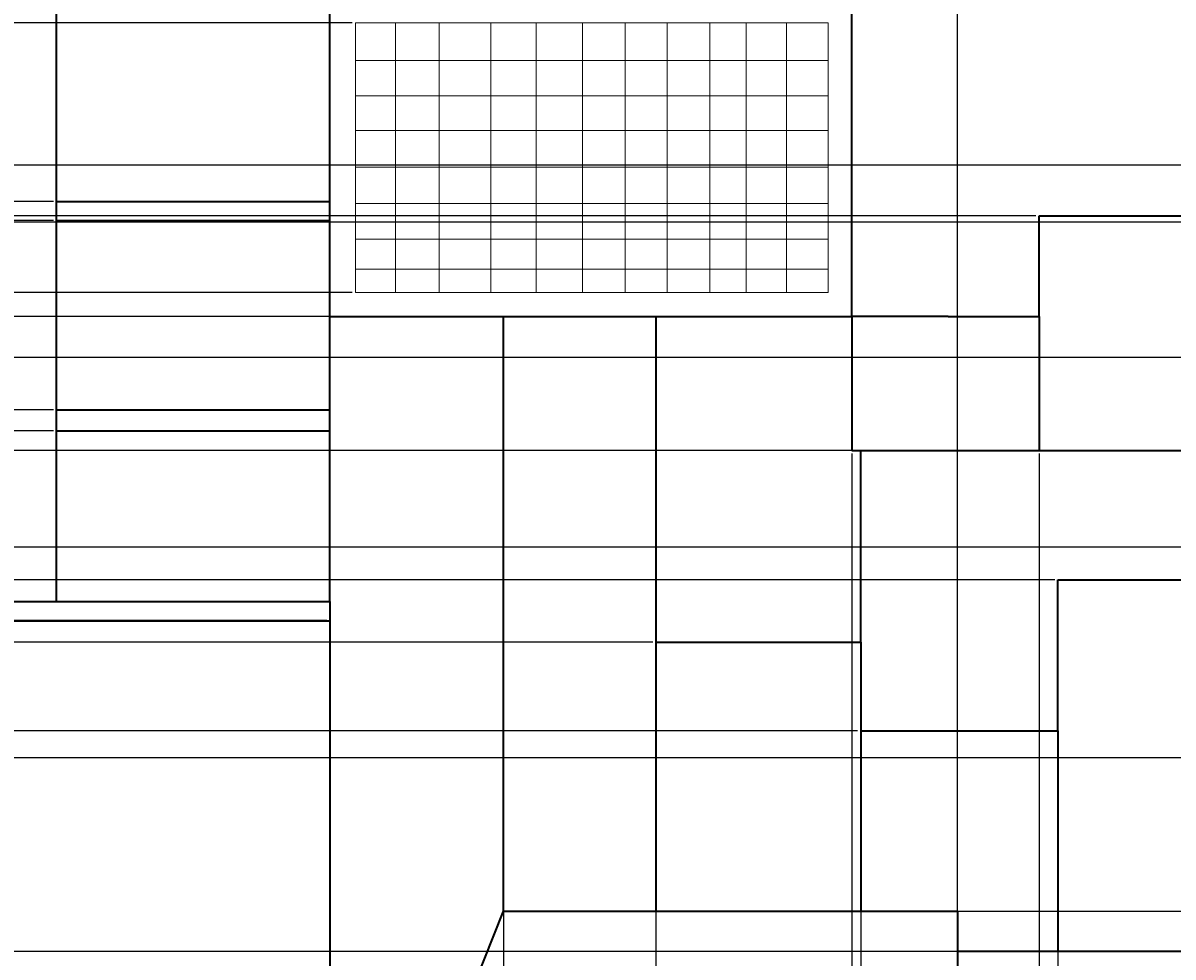
# Model space of a CAD drawing. Units: inches. Extents: x -10 to 130, y -32 to 34.
# Tile 4 of 22: x 25.72 to 49.15, y -13.47 to 5.57. Entities that reach past the tile are written whole.
import ezdxf

# ---------------------------------------------------------------- set-up
doc = ezdxf.new("R2010")
doc.units = ezdxf.units.IN
doc.header["$MEASUREMENT"] = 0
for name, color, linetype, lineweight in [('A-ANNO-DIMS', 2, 'Continuous', 18), ('A-ELEV', 7, 'Continuous', 35), ('A-GLAZ', 4, 'Continuous', 18)]:
    doc.layers.add(name, color=color, linetype=linetype, lineweight=lineweight)
doc.styles.get("Standard").update_dxf_attribs({"font": 'arial.ttf'})
doc.dimstyles.get("Standard").update_dxf_attribs({"dimtxt": 0.18, "dimasz": 0.18, "dimexe": 0.18, "dimexo": 0.0625, "dimgap": 0.09, "dimtad": 0, "dimtih": 1, "dimtoh": 1, "dimdec": 4, "dimzin": 0, "dimdsep": 46, "dimtxsty": 'Standard', "dimcen": 0.09, "dimadec": 0, "dimazin": 0, "dimtfac": 1, "dimtdec": 4, "dimtofl": 0, "dimtmove": 0, "dimatfit": 3, "dimfxl": 1, "dimtolj": 1, "dimtzin": 0, "dimarcsym": 0})

# ---------------------------------------------------------------- blocks, each defined once
blk = doc.blocks.new('*D32')
at = {"layer": 'A-ANNO-DIMS', "color": 0, "lineweight": -2, "transparency": 16777216}
for p, q in [((31.909, -0.414), (-9.564, -0.414)), ((-9.384, -0.594), (-9.384, -3.136)), ((-9.384, -6.042), (-9.384, -3.5)), ((13.34, -6.222), (-9.564, -6.222))]:
    blk.add_line(p, q, dxfattribs=at)
at = {"layer": 'A-ANNO-DIMS', "color": 0, "transparency": 16777216}
for points in [[(-9.414, -0.594), (-9.354, -0.594), (-9.384, -0.414)], [(-9.414, -6.042), (-9.354, -6.042), (-9.384, -6.222)]]:
    blk.add_solid(points, dxfattribs=at)
at = {"layer": 'Defpoints', "color": 0, "transparency": 16777216}
for p in [(-9.384, -0.414), (31.971, -0.414), (13.402, -6.222)]:
    blk.add_point(p, dxfattribs=at)
at = {"layer": 'A-ANNO-DIMS', "color": 0, "transparency": 16777216, "insert": (-9.384, -3.318), "char_height": 0.18, "attachment_point": 5}
blk.add_mtext('\\A1;5.808', dxfattribs=at)
blk = doc.blocks.new('*D33')
at = {"layer": 'A-ANNO-DIMS', "color": 0, "lineweight": -2, "transparency": 16777216}
for p, q in [((70.835, 1.511), (-9.564, 1.511)), ((-9.384, 1.331), (-9.384, 0.73)), ((-9.384, -0.234), (-9.384, 0.367)), ((31.909, -0.414), (-9.564, -0.414))]:
    blk.add_line(p, q, dxfattribs=at)
at = {"layer": 'A-ANNO-DIMS', "color": 0, "transparency": 16777216}
for points in [[(-9.414, 1.331), (-9.354, 1.331), (-9.384, 1.511)], [(-9.414, -0.234), (-9.354, -0.234), (-9.384, -0.414)]]:
    blk.add_solid(points, dxfattribs=at)
at = {"layer": 'Defpoints', "color": 0, "transparency": 16777216}
for p in [(-9.384, 1.511), (70.898, 1.511), (31.971, -0.414)]:
    blk.add_point(p, dxfattribs=at)
at = {"layer": 'A-ANNO-DIMS', "color": 0, "transparency": 16777216, "insert": (-9.384, 0.548), "char_height": 0.18, "attachment_point": 5}
blk.add_mtext('\\A1;1.92', dxfattribs=at)
blk = doc.blocks.new('*D34')
at = {"layer": 'A-ANNO-DIMS', "color": 0, "lineweight": -2, "transparency": 16777216}
for p, q in [((13.34, 6.007), (-9.564, 6.007)), ((-9.384, 5.827), (-9.384, 3.941)), ((-9.384, 1.691), (-9.384, 3.577)), ((70.835, 1.511), (-9.564, 1.511))]:
    blk.add_line(p, q, dxfattribs=at)
at = {"layer": 'A-ANNO-DIMS', "color": 0, "transparency": 16777216}
for points in [[(-9.414, 5.827), (-9.354, 5.827), (-9.384, 6.007)], [(-9.414, 1.691), (-9.354, 1.691), (-9.384, 1.511)]]:
    blk.add_solid(points, dxfattribs=at)
at = {"layer": 'Defpoints', "color": 0, "transparency": 16777216}
for p in [(-9.384, 6.007), (13.402, 6.007), (70.898, 1.511)]:
    blk.add_point(p, dxfattribs=at)
at = {"layer": 'A-ANNO-DIMS', "color": 0, "transparency": 16777216, "insert": (-9.384, 3.759), "char_height": 0.18, "attachment_point": 5}
blk.add_mtext('\\A1;4.497', dxfattribs=at)
blk = doc.blocks.new('*D43')
at = {"layer": 'A-ANNO-DIMS', "color": 0, "lineweight": -2, "transparency": 16777216}
for p, q in [((35.505, -12.596), (35.505, -28.129)), ((31.971, -21.477), (31.971, -28.129)), ((32.151, -27.949), (33.414, -27.949)), ((35.325, -27.949), (34.062, -27.949))]:
    blk.add_line(p, q, dxfattribs=at)
at = {"layer": 'A-ANNO-DIMS', "color": 0, "transparency": 16777216}
for points in [[(32.151, -27.919), (32.151, -27.979), (31.971, -27.949)], [(35.325, -27.919), (35.325, -27.979), (35.505, -27.949)]]:
    blk.add_solid(points, dxfattribs=at)
at = {"layer": 'Defpoints', "color": 0, "transparency": 16777216}
for p in [(35.505, -12.534), (31.971, -21.414), (35.505, -27.949)]:
    blk.add_point(p, dxfattribs=at)
at = {"layer": 'A-ANNO-DIMS', "color": 0, "transparency": 16777216, "insert": (33.738, -27.949), "char_height": 0.18, "attachment_point": 5}
blk.add_mtext('\\A1;3.53', dxfattribs=at)
blk = doc.blocks.new('*D44')
at = {"layer": 'A-ANNO-DIMS', "color": 0, "lineweight": -2, "transparency": 16777216}
for p, q in [((35.505, -12.596), (35.505, -28.129)), ((44.76, -21.477), (44.76, -28.129)), ((35.685, -27.949), (39.738, -27.949)), ((44.58, -27.949), (40.527, -27.949))]:
    blk.add_line(p, q, dxfattribs=at)
at = {"layer": 'A-ANNO-DIMS', "color": 0, "transparency": 16777216}
for points in [[(35.685, -27.919), (35.685, -27.979), (35.505, -27.949)], [(44.58, -27.919), (44.58, -27.979), (44.76, -27.949)]]:
    blk.add_solid(points, dxfattribs=at)
at = {"layer": 'Defpoints', "color": 0, "transparency": 16777216}
for p in [(35.505, -12.534), (44.76, -21.414), (44.76, -27.949)]:
    blk.add_point(p, dxfattribs=at)
at = {"layer": 'A-ANNO-DIMS', "color": 0, "transparency": 16777216, "insert": (40.132, -27.949), "char_height": 0.18, "attachment_point": 5}
blk.add_mtext('\\A1;9.255', dxfattribs=at)
blk = doc.blocks.new('*D47')
at = {"layer": 'A-ANNO-DIMS', "color": 0, "lineweight": -2, "transparency": 16777216}
for p, q in [((35.567, -12.534), (129.508, -12.534)), ((129.328, -12.714), (129.328, -16.792)), ((129.328, -21.234), (129.328, -17.156)), ((32.034, -21.414), (129.508, -21.414))]:
    blk.add_line(p, q, dxfattribs=at)
at = {"layer": 'A-ANNO-DIMS', "color": 0, "transparency": 16777216}
for points in [[(129.298, -12.714), (129.358, -12.714), (129.328, -12.534)], [(129.298, -21.234), (129.358, -21.234), (129.328, -21.414)]]:
    blk.add_solid(points, dxfattribs=at)
at = {"layer": 'Defpoints', "color": 0, "transparency": 16777216}
for p in [(35.505, -12.534), (31.971, -21.414), (129.328, -21.414)]:
    blk.add_point(p, dxfattribs=at)
at = {"layer": 'A-ANNO-DIMS', "color": 0, "transparency": 16777216, "insert": (129.328, -16.974), "char_height": 0.18, "attachment_point": 5}
blk.add_mtext('\\A1;8.88', dxfattribs=at)
blk = doc.blocks.new('*D48')
at = {"layer": 'A-ANNO-DIMS', "color": 0, "lineweight": -2, "transparency": 16777216}
for p, q in [((44.76, -13.293), (44.76, 33.879)), ((74.492, -13.293), (74.492, 33.879)), ((44.94, 33.699), (59.231, 33.699)), ((74.312, 33.699), (60.021, 33.699))]:
    blk.add_line(p, q, dxfattribs=at)
at = {"layer": 'A-ANNO-DIMS', "color": 0, "transparency": 16777216}
for points in [[(44.94, 33.729), (44.94, 33.669), (44.76, 33.699)], [(74.312, 33.729), (74.312, 33.669), (74.492, 33.699)]]:
    blk.add_solid(points, dxfattribs=at)
at = {"layer": 'Defpoints', "color": 0, "transparency": 16777216}
for p in [(74.492, 33.699), (44.76, -13.356), (74.492, -13.356)]:
    blk.add_point(p, dxfattribs=at)
at = {"layer": 'A-ANNO-DIMS', "color": 0, "transparency": 16777216, "insert": (59.626, 33.699), "char_height": 0.18, "attachment_point": 5}
blk.add_mtext('\\A1;29.73', dxfattribs=at)
blk = doc.blocks.new('*D49')
at = {"layer": 'A-ANNO-DIMS', "color": 0, "lineweight": -2, "transparency": 16777216}
for p, q in [((44.697, -13.356), (-9.564, -13.356)), ((-9.384, -13.536), (-9.384, -17.203)), ((-9.384, -21.234), (-9.384, -17.567)), ((44.697, -21.414), (-9.564, -21.414))]:
    blk.add_line(p, q, dxfattribs=at)
at = {"layer": 'A-ANNO-DIMS', "color": 0, "transparency": 16777216}
for points in [[(-9.414, -13.536), (-9.354, -13.536), (-9.384, -13.356)], [(-9.414, -21.234), (-9.354, -21.234), (-9.384, -21.414)]]:
    blk.add_solid(points, dxfattribs=at)
at = {"layer": 'Defpoints', "color": 0, "transparency": 16777216}
for p in [(44.76, -13.356), (-9.384, -21.414), (44.76, -21.414)]:
    blk.add_point(p, dxfattribs=at)
at = {"layer": 'A-ANNO-DIMS', "color": 0, "transparency": 16777216, "insert": (-9.384, -17.385), "char_height": 0.18, "attachment_point": 5}
blk.add_mtext('\\A1;8.059', dxfattribs=at)
blk = doc.blocks.new('*D90')
at = {"layer": 'A-ANNO-DIMS', "color": 0, "lineweight": -2, "transparency": 16777216}
for p, q in [((49.884, 5.802), (-9.564, 5.802)), ((-9.384, 5.622), (-9.384, 4.421)), ((-9.384, 2.855), (-9.384, 4.057)), ((49.884, 2.675), (-9.564, 2.675))]:
    blk.add_line(p, q, dxfattribs=at)
at = {"layer": 'A-ANNO-DIMS', "color": 0, "transparency": 16777216}
for points in [[(-9.414, 5.622), (-9.354, 5.622), (-9.384, 5.802)], [(-9.414, 2.855), (-9.354, 2.855), (-9.384, 2.675)]]:
    blk.add_solid(points, dxfattribs=at)
at = {"layer": 'Defpoints', "color": 0, "transparency": 16777216}
for p in [(49.946, 5.802), (-9.384, 2.675), (49.946, 2.675)]:
    blk.add_point(p, dxfattribs=at)
at = {"layer": 'A-ANNO-DIMS', "color": 0, "transparency": 16777216, "insert": (-9.384, 4.239), "char_height": 0.18, "attachment_point": 5}
blk.add_mtext('\\A1;3.127', dxfattribs=at)
blk = doc.blocks.new('*D91')
at = {"layer": 'A-ANNO-DIMS', "color": 0, "lineweight": -2, "transparency": 16777216}
for p, q in [((49.884, 2.675), (-9.564, 2.675)), ((-9.384, 2.495), (-9.384, 0.895)), ((-9.384, -1.07), (-9.384, 0.531)), ((49.884, -1.25), (-9.564, -1.25))]:
    blk.add_line(p, q, dxfattribs=at)
at = {"layer": 'A-ANNO-DIMS', "color": 0, "transparency": 16777216}
for points in [[(-9.414, 2.495), (-9.354, 2.495), (-9.384, 2.675)], [(-9.414, -1.07), (-9.354, -1.07), (-9.384, -1.25)]]:
    blk.add_solid(points, dxfattribs=at)
at = {"layer": 'Defpoints', "color": 0, "transparency": 16777216}
for p in [(49.946, 2.675), (-9.384, -1.25), (49.946, -1.25)]:
    blk.add_point(p, dxfattribs=at)
at = {"layer": 'A-ANNO-DIMS', "color": 0, "transparency": 16777216, "insert": (-9.384, 0.713), "char_height": 0.18, "attachment_point": 5}
blk.add_mtext('\\A1;3.925', dxfattribs=at)
blk = doc.blocks.new('*D92')
at = {"layer": 'A-ANNO-DIMS', "color": 0, "lineweight": -2, "transparency": 16777216}
for p, q in [((49.884, -1.25), (-9.564, -1.25)), ((-9.384, -1.43), (-9.384, -3.001)), ((-9.384, -4.936), (-9.384, -3.365)), ((49.884, -5.116), (-9.564, -5.116))]:
    blk.add_line(p, q, dxfattribs=at)
at = {"layer": 'A-ANNO-DIMS', "color": 0, "transparency": 16777216}
for points in [[(-9.414, -1.43), (-9.354, -1.43), (-9.384, -1.25)], [(-9.414, -4.936), (-9.354, -4.936), (-9.384, -5.116)]]:
    blk.add_solid(points, dxfattribs=at)
at = {"layer": 'Defpoints', "color": 0, "transparency": 16777216}
for p in [(49.946, -1.25), (-9.384, -5.116), (49.946, -5.116)]:
    blk.add_point(p, dxfattribs=at)
at = {"layer": 'A-ANNO-DIMS', "color": 0, "transparency": 16777216, "insert": (-9.384, -3.183), "char_height": 0.18, "attachment_point": 5}
blk.add_mtext('\\A1;3.866', dxfattribs=at)
blk = doc.blocks.new('*D93')
at = {"layer": 'A-ANNO-DIMS', "color": 0, "lineweight": -2, "transparency": 16777216}
for p, q in [((49.884, -5.116), (-9.564, -5.116)), ((-9.384, -5.296), (-9.384, -7.081)), ((-9.384, -9.23), (-9.384, -7.445)), ((49.884, -9.41), (-9.564, -9.41))]:
    blk.add_line(p, q, dxfattribs=at)
at = {"layer": 'A-ANNO-DIMS', "color": 0, "transparency": 16777216}
for points in [[(-9.414, -5.296), (-9.354, -5.296), (-9.384, -5.116)], [(-9.414, -9.23), (-9.354, -9.23), (-9.384, -9.41)]]:
    blk.add_solid(points, dxfattribs=at)
at = {"layer": 'Defpoints', "color": 0, "transparency": 16777216}
for p in [(49.946, -5.116), (-9.384, -9.41), (49.946, -9.41)]:
    blk.add_point(p, dxfattribs=at)
at = {"layer": 'A-ANNO-DIMS', "color": 0, "transparency": 16777216, "insert": (-9.384, -7.263), "char_height": 0.18, "attachment_point": 5}
blk.add_mtext('\\A1;4.294', dxfattribs=at)
blk = doc.blocks.new('*D94')
at = {"layer": 'A-ANNO-DIMS', "color": 0, "lineweight": -2, "transparency": 16777216}
for p, q in [((49.884, -9.41), (-9.564, -9.41)), ((-9.384, -9.59), (-9.384, -11.201)), ((-9.384, -13.176), (-9.384, -11.565)), ((49.884, -13.356), (-9.564, -13.356))]:
    blk.add_line(p, q, dxfattribs=at)
at = {"layer": 'A-ANNO-DIMS', "color": 0, "transparency": 16777216}
for points in [[(-9.414, -9.59), (-9.354, -9.59), (-9.384, -9.41)], [(-9.414, -13.176), (-9.354, -13.176), (-9.384, -13.356)]]:
    blk.add_solid(points, dxfattribs=at)
at = {"layer": 'Defpoints', "color": 0, "transparency": 16777216}
for p in [(49.946, -9.41), (-9.384, -13.356), (49.946, -13.356)]:
    blk.add_point(p, dxfattribs=at)
at = {"layer": 'A-ANNO-DIMS', "color": 0, "transparency": 16777216, "insert": (-9.384, -11.383), "char_height": 0.18, "attachment_point": 5}
blk.add_mtext('\\A1;3.946', dxfattribs=at)
blk = doc.blocks.new('*D115')
at = {"layer": 'A-ANNO-DIMS', "color": 0, "lineweight": -2, "transparency": 16777216}
for p, q in [((26.336, 6.007), (-9.564, 6.007)), ((-9.384, 5.827), (-9.384, 4.151)), ((-9.384, 2.111), (-9.384, 3.787)), ((26.336, 1.931), (-9.564, 1.931))]:
    blk.add_line(p, q, dxfattribs=at)
at = {"layer": 'A-ANNO-DIMS', "color": 0, "transparency": 16777216}
for points in [[(-9.414, 5.827), (-9.354, 5.827), (-9.384, 6.007)], [(-9.414, 2.111), (-9.354, 2.111), (-9.384, 1.931)]]:
    blk.add_solid(points, dxfattribs=at)
at = {"layer": 'Defpoints', "color": 0, "transparency": 16777216}
for p in [(26.399, 6.007), (-9.384, 1.931), (26.399, 1.931)]:
    blk.add_point(p, dxfattribs=at)
at = {"layer": 'A-ANNO-DIMS', "color": 0, "transparency": 16777216, "insert": (-9.384, 3.969), "char_height": 0.18, "attachment_point": 5}
blk.add_mtext('\\A1;4.076', dxfattribs=at)
blk = doc.blocks.new('*D116')
at = {"layer": 'A-ANNO-DIMS', "color": 0, "lineweight": -2, "transparency": 16777216}
for p, q in [((-9.383551, 2.111013), (-9.383551, 2.291013)), ((26.336278, 1.931013), (-9.563551, 1.931013)), ((26.336278, 1.544827), (-9.563551, 1.544827)), ((-9.383551, 1.364827), (-9.383551, 1.184827))]:
    blk.add_line(p, q, dxfattribs=at)
at = {"layer": 'A-ANNO-DIMS', "color": 0, "transparency": 16777216}
for points in [[(-9.413551, 2.111013), (-9.353551, 2.111013), (-9.383551, 1.931013)], [(-9.413551, 1.364827), (-9.353551, 1.364827), (-9.383551, 1.544827)]]:
    blk.add_solid(points, dxfattribs=at)
at = {"layer": 'Defpoints', "color": 0, "transparency": 16777216}
for p in [(26.398778, 1.931013), (-9.383551, 1.544827), (26.398778, 1.544827)]:
    blk.add_point(p, dxfattribs=at)
at = {"layer": 'A-ANNO-DIMS', "color": 0, "transparency": 16777216, "insert": (-9.383551, 1.73792), "char_height": 0.18, "attachment_point": 5}
blk.add_mtext('\\A1;0.386', dxfattribs=at)
blk = doc.blocks.new('*D117')
at = {"layer": 'A-ANNO-DIMS', "color": 0, "lineweight": -2, "transparency": 16777216}
for p, q in [((26.336, 1.545), (-9.564, 1.545)), ((-9.384, 1.365), (-9.384, -0.204)), ((-9.384, -2.137), (-9.384, -0.568)), ((26.336, -2.317), (-9.564, -2.317))]:
    blk.add_line(p, q, dxfattribs=at)
at = {"layer": 'A-ANNO-DIMS', "color": 0, "transparency": 16777216}
for points in [[(-9.414, 1.365), (-9.354, 1.365), (-9.384, 1.545)], [(-9.414, -2.137), (-9.354, -2.137), (-9.384, -2.317)]]:
    blk.add_solid(points, dxfattribs=at)
at = {"layer": 'Defpoints', "color": 0, "transparency": 16777216}
for p in [(26.399, 1.545), (-9.384, -2.317), (26.399, -2.317)]:
    blk.add_point(p, dxfattribs=at)
at = {"layer": 'A-ANNO-DIMS', "color": 0, "transparency": 16777216, "insert": (-9.384, -0.386), "char_height": 0.18, "attachment_point": 5}
blk.add_mtext('\\A1;3.862', dxfattribs=at)
blk = doc.blocks.new('*D118')
at = {"layer": 'A-ANNO-DIMS', "color": 0, "lineweight": -2, "transparency": 16777216}
for p, q in [((-9.384, -2.137), (-9.384, -1.957)), ((26.336, -2.317), (-9.564, -2.317)), ((26.336, -2.746), (-9.564, -2.746)), ((-9.384, -2.926), (-9.384, -3.106))]:
    blk.add_line(p, q, dxfattribs=at)
at = {"layer": 'A-ANNO-DIMS', "color": 0, "transparency": 16777216}
for points in [[(-9.414, -2.137), (-9.354, -2.137), (-9.384, -2.317)], [(-9.414, -2.926), (-9.354, -2.926), (-9.384, -2.746)]]:
    blk.add_solid(points, dxfattribs=at)
at = {"layer": 'Defpoints', "color": 0, "transparency": 16777216}
for p in [(26.399, -2.317), (-9.384, -2.746), (26.399, -2.746)]:
    blk.add_point(p, dxfattribs=at)
at = {"layer": 'A-ANNO-DIMS', "color": 0, "transparency": 16777216, "insert": (-9.384, -2.532), "char_height": 0.18, "attachment_point": 5}
blk.add_mtext('\\A1;0.429', dxfattribs=at)
blk = doc.blocks.new('*D121')
at = {"layer": 'A-ANNO-DIMS', "color": 0, "lineweight": -2, "transparency": 16777216}
for p, q in [((-9.384, 6.187), (-9.384, 6.367)), ((31.909, 6.007), (-9.564, 6.007)), ((32.427, 5.572), (-9.564, 5.572)), ((-9.384, 5.392), (-9.384, 5.212))]:
    blk.add_line(p, q, dxfattribs=at)
at = {"layer": 'A-ANNO-DIMS', "color": 0, "transparency": 16777216}
for points in [[(-9.414, 6.187), (-9.354, 6.187), (-9.384, 6.007)], [(-9.414, 5.392), (-9.354, 5.392), (-9.384, 5.572)]]:
    blk.add_solid(points, dxfattribs=at)
at = {"layer": 'Defpoints', "color": 0, "transparency": 16777216}
for p in [(-9.384, 6.007), (31.971, 6.007), (32.49, 5.572)]:
    blk.add_point(p, dxfattribs=at)
at = {"layer": 'A-ANNO-DIMS', "color": 0, "transparency": 16777216, "insert": (-9.384, 5.789), "char_height": 0.18, "attachment_point": 5}
blk.add_mtext('\\A1;0.436', dxfattribs=at)
blk = doc.blocks.new('*D122')
at = {"layer": 'A-ANNO-DIMS', "color": 0, "lineweight": -2, "transparency": 16777216}
for p, q in [((-9.383551, 0.25916), (-9.383551, 0.43916)), ((32.427309, 0.07916), (-9.563551, 0.07916)), ((31.908661, -0.413828), (-9.563551, -0.413828)), ((-9.383551, -0.593828), (-9.383551, -0.773828))]:
    blk.add_line(p, q, dxfattribs=at)
at = {"layer": 'A-ANNO-DIMS', "color": 0, "transparency": 16777216}
for points in [[(-9.413551, 0.25916), (-9.353551, 0.25916), (-9.383551, 0.07916)], [(-9.413551, -0.593828), (-9.353551, -0.593828), (-9.383551, -0.413828)]]:
    blk.add_solid(points, dxfattribs=at)
at = {"layer": 'Defpoints', "color": 0, "transparency": 16777216}
for p in [(32.489809, 0.07916), (-9.383551, -0.413828), (31.971161, -0.413828)]:
    blk.add_point(p, dxfattribs=at)
at = {"layer": 'A-ANNO-DIMS', "color": 0, "transparency": 16777216, "insert": (-9.383551, -0.167334), "char_height": 0.18, "attachment_point": 5}
blk.add_mtext('\\A1;0.493', dxfattribs=at)
blk = doc.blocks.new('*D123')
at = {"layer": 'A-ANNO-DIMS', "color": 0, "lineweight": -2, "transparency": 16777216}
for p, q in [((35.505, -0.476), (35.505, -28.129)), ((38.612, -0.476), (38.612, -28.129)), ((35.685, -27.949), (36.665, -27.949)), ((38.432, -27.949), (37.452, -27.949))]:
    blk.add_line(p, q, dxfattribs=at)
at = {"layer": 'A-ANNO-DIMS', "color": 0, "transparency": 16777216}
for points in [[(35.685, -27.919), (35.685, -27.979), (35.505, -27.949)], [(38.432, -27.919), (38.432, -27.979), (38.612, -27.949)]]:
    blk.add_solid(points, dxfattribs=at)
at = {"layer": 'Defpoints', "color": 0, "transparency": 16777216}
for p in [(35.505, -0.414), (38.612, -0.414), (38.612, -27.949)]:
    blk.add_point(p, dxfattribs=at)
at = {"layer": 'A-ANNO-DIMS', "color": 0, "transparency": 16777216, "insert": (37.058, -27.949), "char_height": 0.18, "attachment_point": 5}
blk.add_mtext('\\A1;3.108', dxfattribs=at)
blk = doc.blocks.new('*D124')
at = {"layer": 'A-ANNO-DIMS', "color": 0, "lineweight": -2, "transparency": 16777216}
for p, q in [((38.612, -7.112), (38.612, -28.129)), ((42.788, -7.112), (42.788, -28.129)), ((38.792, -27.949), (40.303, -27.949)), ((42.608, -27.949), (41.097, -27.949))]:
    blk.add_line(p, q, dxfattribs=at)
at = {"layer": 'A-ANNO-DIMS', "color": 0, "transparency": 16777216}
for points in [[(38.792, -27.919), (38.792, -27.979), (38.612, -27.949)], [(42.608, -27.919), (42.608, -27.979), (42.788, -27.949)]]:
    blk.add_solid(points, dxfattribs=at)
at = {"layer": 'Defpoints', "color": 0, "transparency": 16777216}
for p in [(38.612, -7.05), (42.788, -7.05), (42.788, -27.949)]:
    blk.add_point(p, dxfattribs=at)
at = {"layer": 'A-ANNO-DIMS', "color": 0, "transparency": 16777216, "insert": (40.7, -27.949), "char_height": 0.18, "attachment_point": 5}
blk.add_mtext('\\A1;4.176', dxfattribs=at)
blk = doc.blocks.new('*D125')
at = {"layer": 'A-ANNO-DIMS', "color": 0, "lineweight": -2, "transparency": 16777216}
for p, q in [((38.55, -0.414), (-9.564, -0.414)), ((-9.384, -0.594), (-9.384, -3.55)), ((-9.384, -6.87), (-9.384, -3.914)), ((38.55, -7.05), (-9.564, -7.05))]:
    blk.add_line(p, q, dxfattribs=at)
at = {"layer": 'A-ANNO-DIMS', "color": 0, "transparency": 16777216}
for points in [[(-9.414, -0.594), (-9.354, -0.594), (-9.384, -0.414)], [(-9.414, -6.87), (-9.354, -6.87), (-9.384, -7.05)]]:
    blk.add_solid(points, dxfattribs=at)
at = {"layer": 'Defpoints', "color": 0, "transparency": 16777216}
for p in [(38.612, -0.414), (-9.384, -7.05), (38.612, -7.05)]:
    blk.add_point(p, dxfattribs=at)
at = {"layer": 'A-ANNO-DIMS', "color": 0, "transparency": 16777216, "insert": (-9.384, -3.732), "char_height": 0.18, "attachment_point": 5}
blk.add_mtext('\\A1;6.636', dxfattribs=at)
blk = doc.blocks.new('*D126')
at = {"layer": 'A-ANNO-DIMS', "color": 0, "lineweight": -2, "transparency": 16777216}
for p, q in [((42.609, -3.206), (42.609, -28.129)), ((46.423, -3.206), (46.423, -28.129)), ((42.789, -27.949), (44.123, -27.949)), ((46.243, -27.949), (44.909, -27.949))]:
    blk.add_line(p, q, dxfattribs=at)
at = {"layer": 'A-ANNO-DIMS', "color": 0, "transparency": 16777216}
for points in [[(42.789, -27.919), (42.789, -27.979), (42.609, -27.949)], [(46.243, -27.919), (46.243, -27.979), (46.423, -27.949)]]:
    blk.add_solid(points, dxfattribs=at)
at = {"layer": 'Defpoints', "color": 0, "transparency": 16777216}
for p in [(42.609, -3.144), (46.423, -3.144), (46.423, -27.949)]:
    blk.add_point(p, dxfattribs=at)
at = {"layer": 'A-ANNO-DIMS', "color": 0, "transparency": 16777216, "insert": (44.516, -27.949), "char_height": 0.18, "attachment_point": 5}
blk.add_mtext('\\A1;3.814', dxfattribs=at)
blk = doc.blocks.new('*D127')
at = {"layer": 'A-ANNO-DIMS', "color": 0, "lineweight": -2, "transparency": 16777216}
for p, q in [((46.36, 1.642), (-9.564, 1.642)), ((-9.384, 1.462), (-9.384, -0.569)), ((-9.384, -2.964), (-9.384, -0.933)), ((46.36, -3.144), (-9.564, -3.144))]:
    blk.add_line(p, q, dxfattribs=at)
at = {"layer": 'A-ANNO-DIMS', "color": 0, "transparency": 16777216}
for points in [[(-9.414, 1.462), (-9.354, 1.462), (-9.384, 1.642)], [(-9.414, -2.964), (-9.354, -2.964), (-9.384, -3.144)]]:
    blk.add_solid(points, dxfattribs=at)
at = {"layer": 'Defpoints', "color": 0, "transparency": 16777216}
for p in [(46.423, 1.642), (-9.384, -3.144), (46.423, -3.144)]:
    blk.add_point(p, dxfattribs=at)
at = {"layer": 'A-ANNO-DIMS', "color": 0, "transparency": 16777216, "insert": (-9.384, -0.751), "char_height": 0.18, "attachment_point": 5}
blk.add_mtext('\\A1;4.786', dxfattribs=at)
blk = doc.blocks.new('*D128')
at = {"layer": 'A-ANNO-DIMS', "color": 0, "lineweight": -2, "transparency": 16777216}
for p, q in [((42.788, -8.923), (42.788, -28.129)), ((46.809, -8.923), (46.809, -28.129)), ((42.968, -27.949), (44.419, -27.949)), ((46.629, -27.949), (45.178, -27.949))]:
    blk.add_line(p, q, dxfattribs=at)
at = {"layer": 'A-ANNO-DIMS', "color": 0, "transparency": 16777216}
for points in [[(42.968, -27.919), (42.968, -27.979), (42.788, -27.949)], [(46.629, -27.919), (46.629, -27.979), (46.809, -27.949)]]:
    blk.add_solid(points, dxfattribs=at)
at = {"layer": 'Defpoints', "color": 0, "transparency": 16777216}
for p in [(42.788, -8.861), (46.809, -8.861), (46.809, -27.949)]:
    blk.add_point(p, dxfattribs=at)
at = {"layer": 'A-ANNO-DIMS', "color": 0, "transparency": 16777216, "insert": (44.798, -27.949), "char_height": 0.18, "attachment_point": 5}
blk.add_mtext('\\A1;4.021', dxfattribs=at)
blk = doc.blocks.new('*D129')
at = {"layer": 'A-ANNO-DIMS', "color": 0, "lineweight": -2, "transparency": 16777216}
for p, q in [((42.726, -3.144), (-9.564, -3.144)), ((-9.384, -3.324), (-9.384, -5.82)), ((-9.384, -8.681), (-9.384, -6.184)), ((42.726, -8.861), (-9.564, -8.861))]:
    blk.add_line(p, q, dxfattribs=at)
at = {"layer": 'A-ANNO-DIMS', "color": 0, "transparency": 16777216}
for points in [[(-9.414, -3.324), (-9.354, -3.324), (-9.384, -3.144)], [(-9.414, -8.681), (-9.354, -8.681), (-9.384, -8.861)]]:
    blk.add_solid(points, dxfattribs=at)
at = {"layer": 'Defpoints', "color": 0, "transparency": 16777216}
for p in [(42.788, -3.144), (-9.384, -8.861), (42.788, -8.861)]:
    blk.add_point(p, dxfattribs=at)
at = {"layer": 'A-ANNO-DIMS', "color": 0, "transparency": 16777216, "insert": (-9.384, -6.002), "char_height": 0.18, "attachment_point": 5}
blk.add_mtext('\\A1;5.717', dxfattribs=at)
blk = doc.blocks.new('*D130')
at = {"layer": 'A-ANNO-DIMS', "color": 0, "lineweight": -2, "transparency": 16777216}
for p, q in [((46.746, -5.784), (-9.564, -5.784)), ((-9.384, -5.964), (-9.384, -9.388)), ((-9.384, -13.176), (-9.384, -9.752)), ((46.746, -13.356), (-9.564, -13.356))]:
    blk.add_line(p, q, dxfattribs=at)
at = {"layer": 'A-ANNO-DIMS', "color": 0, "transparency": 16777216}
for points in [[(-9.414, -5.964), (-9.354, -5.964), (-9.384, -5.784)], [(-9.414, -13.176), (-9.354, -13.176), (-9.384, -13.356)]]:
    blk.add_solid(points, dxfattribs=at)
at = {"layer": 'Defpoints', "color": 0, "transparency": 16777216}
for p in [(46.809, -5.784), (-9.384, -13.356), (46.809, -13.356)]:
    blk.add_point(p, dxfattribs=at)
at = {"layer": 'A-ANNO-DIMS', "color": 0, "transparency": 16777216, "insert": (-9.384, -9.57), "char_height": 0.18, "attachment_point": 5}
blk.add_mtext('\\A1;7.572', dxfattribs=at)
blk = doc.blocks.new('*D131')
at = {"layer": 'A-ANNO-DIMS', "color": 0, "lineweight": -2, "transparency": 16777216}
for p, q in [((-9.384, -6.042), (-9.384, -5.862)), ((31.909, -6.222), (-9.564, -6.222)), ((31.909, -6.613), (-9.564, -6.613)), ((-9.384, -6.793), (-9.384, -6.973))]:
    blk.add_line(p, q, dxfattribs=at)
at = {"layer": 'A-ANNO-DIMS', "color": 0, "transparency": 16777216}
for points in [[(-9.414, -6.042), (-9.354, -6.042), (-9.384, -6.222)], [(-9.414, -6.793), (-9.354, -6.793), (-9.384, -6.613)]]:
    blk.add_solid(points, dxfattribs=at)
at = {"layer": 'Defpoints', "color": 0, "transparency": 16777216}
for p in [(31.971, -6.222), (-9.384, -6.613), (31.971, -6.613)]:
    blk.add_point(p, dxfattribs=at)
at = {"layer": 'A-ANNO-DIMS', "color": 0, "transparency": 16777216, "insert": (-9.384, -6.417), "char_height": 0.18, "attachment_point": 5}
blk.add_mtext('\\A1;0.391', dxfattribs=at)

msp = doc.modelspace()

# ---------------------------------------------------------------- linework, layer by layer
at = {"layer": 'A-ELEV'}
for p, q in [((26.3988, -6.2218), (26.3988, 6.0074)), ((31.9712, -6.2218), (31.9712, 6.0074)), ((42.6089, -0.4138), (42.6089, 6.0074)), ((26.3988, 1.931), (31.9712, 1.931)), ((46.4227, -0.4138), (46.4227, 1.6419)), ((46.4227, 1.6419), (49.9462, 1.6419)), ((26.3988, 1.5448), (31.9712, 1.5448)), ((31.9712, -0.4138), (42.6089, -0.4138)), ((35.5046, -0.4138), (35.5046, -12.5339)), ((38.6123, -0.4138), (38.6123, -12.5339)), ((44.5688, -0.4138), (42.6089, -0.4138)), ((42.6089, -0.4138), (42.6089, -3.1438)), ((44.5688, -0.4138), (46.4227, -0.4138)), ((46.4227, -0.4138), (46.4227, -3.1438)), ((26.3988, -2.317), (31.9712, -2.317)), ((26.3988, -2.7461), (31.9712, -2.7461)), ((42.6089, -3.1438), (42.7881, -3.1438)), ((42.7881, -7.05), (42.7881, -3.1438)), ((42.7881, -3.1438), (49.9462, -3.1438)), ((46.8089, -8.8608), (46.8089, -5.7836)), ((46.8089, -5.7836), (49.9462, -5.7836)), ((13.4021, -6.2218), (26.3988, -6.2218)), ((26.3988, -6.2218), (31.9712, -6.2218)), ((31.9712, -6.2218), (31.9712, -16.1883)), ((21.1687, -6.6131), (26.3988, -6.6131)), ((26.3988, -6.6131), (31.9712, -6.6131)), ((38.6123, -7.05), (42.7881, -7.05)), ((42.7881, -7.05), (42.7881, -12.5339)), ((42.7881, -8.8608), (46.8089, -8.8608)), ((46.8089, -8.8608), (46.8089, -13.3558)), ((35.5046, -12.5339), (31.9712, -21.4145)), ((35.5046, -12.5339), (38.6123, -12.5339)), ((38.6123, -12.5339), (44.76, -12.5339)), ((44.76, -12.5339), (44.76, -13.3558)), ((54.1471, -13.3558), (44.76, -13.3558)), ((44.76, -13.3558), (44.76, -21.4145))]:
    msp.add_line(p, q, dxfattribs=at)
at = {"layer": 'A-GLAZ'}
for p, q in [((32.4898, 0.0792), (32.4898, 5.5715)), ((32.4898, 5.5715), (42.1266, 5.5715)), ((33.3065, 5.5715), (33.3065, 0.0792)), ((34.1958, 5.5715), (34.1958, 0.0792)), ((35.2484, 5.5715), (35.2484, 0.0792)), ((36.1739, 5.5715), (36.1739, 0.0792)), ((37.1177, 5.5715), (37.1177, 0.0792)), ((37.9888, 5.5715), (37.9888, 0.0792)), ((38.8418, 5.5715), (38.8418, 0.0792)), ((39.7129, 5.5715), (39.7129, 0.0792)), ((40.457, 5.5715), (40.457, 0.0792)), ((41.2736, 5.5715), (41.2736, 0.0792)), ((42.1266, 5.5715), (42.1266, 0.0792)), ((32.4898, 4.8102), (42.1266, 4.8102)), ((32.4898, 4.0852), (42.1266, 4.0852)), ((32.4898, 3.3782), (42.1266, 3.3782)), ((32.4898, 2.635), (42.1266, 2.635)), ((32.4898, 1.8918), (42.1266, 1.8918)), ((32.4898, 1.1668), (42.1266, 1.1668)), ((32.4898, 0.5505), (42.1266, 0.5505)), ((32.4898, 0.0792), (42.1266, 0.0792))]:
    msp.add_line(p, q, dxfattribs=at)

# ---------------------------------------------------------------- dimensions: what is measured, and where the dimension line sits
at = {"layer": 'A-ANNO-DIMS'}
for base, p1, p2, override, picture, middle in [((74.492, 33.6987), (44.76, -13.3558), (74.492, -13.3558), {"dimdec": 2, "dimlfac": 1, "dimrnd": 0, "dimzin": 0, "dimdsep": 46, "dimlunit": 2}, '*D48', (59.626, 33.6987)), ((38.6123, -27.9493), (35.5046, -0.4138), (38.6123, -0.4138), {"dimdec": 3, "dimlfac": 1, "dimrnd": 0, "dimzin": 0, "dimdsep": 46, "dimlunit": 2}, '*D123', (37.0585, -27.9493)), ((46.4227, -27.9493), (42.6089, -3.1438), (46.4227, -3.1438), {"dimdec": 3, "dimlfac": 1, "dimrnd": 0, "dimzin": 0, "dimdsep": 46, "dimlunit": 2}, '*D126', (44.5158, -27.9493)), ((42.7881, -27.9493), (38.6123, -7.05), (42.7881, -7.05), {"dimdec": 3, "dimlfac": 1, "dimrnd": 0, "dimzin": 0, "dimdsep": 46, "dimlunit": 2}, '*D124', (40.7002, -27.9493)), ((46.8089, -27.9493), (42.7881, -8.8608), (46.8089, -8.8608), {"dimdec": 3, "dimlfac": 1, "dimrnd": 0, "dimzin": 0, "dimdsep": 46, "dimlunit": 2}, '*D128', (44.7985, -27.9493)), ((35.5046, -27.9493), (31.9712, -21.4145), (35.5046, -12.5339), {"dimdec": 2, "dimlfac": 1, "dimrnd": 0, "dimzin": 0, "dimdsep": 46, "dimlunit": 2}, '*D43', (33.7379, -27.9493)), ((44.76, -27.9493), (35.5046, -12.5339), (44.76, -21.4145), {"dimdec": 3, "dimlfac": 1, "dimrnd": 0, "dimzin": 0, "dimdsep": 46, "dimlunit": 2}, '*D44', (40.1323, -27.9493))]:
    dim = msp.add_linear_dim(base=base, p1=p1, p2=p2, dimstyle='Standard', override=override, dxfattribs=at)
    dim.commit()
    dim.dimension.update_dxf_attribs({"geometry": picture, "text_midpoint": middle})
for base, p1, p2, override, picture, middle in [((-9.3836, 6.0074), (32.4898, 5.5715), (31.9712, 6.0074), {"dimdec": 3, "dimlfac": 1, "dimrnd": 0, "dimzin": 0, "dimdsep": 46, "dimlunit": 2}, '*D121', (-9.3836, 5.7895)), ((-9.3836, 6.0074), (70.898, 1.5107), (13.4021, 6.0074), {"dimdec": 3, "dimlfac": 1, "dimrnd": 0, "dimzin": 0, "dimdsep": 46, "dimlunit": 2}, '*D34', (-9.3836, 3.7591)), ((-9.3836, 1.931), (26.3988, 6.0074), (26.3988, 1.931), {"dimdec": 3, "dimlfac": 1, "dimrnd": 0, "dimzin": 0, "dimdsep": 46, "dimlunit": 2}, '*D115', (-9.3836, 3.9692)), ((-9.3836, 2.6753), (49.9462, 5.8024), (49.9462, 2.6753), {"dimdec": 3, "dimlfac": 1, "dimrnd": 0, "dimzin": 0, "dimdsep": 46, "dimlunit": 2}, '*D90', (-9.3836, 4.2388)), ((-9.3836, -1.2496), (49.9462, 2.6753), (49.9462, -1.2496), {"dimdec": 3, "dimlfac": 1, "dimrnd": 0, "dimzin": 0, "dimdsep": 46, "dimlunit": 2}, '*D91', (-9.3836, 0.7128)), ((-9.3836, 1.5448), (26.3988, 1.931), (26.3988, 1.5448), {"dimdec": 3, "dimlfac": 1, "dimrnd": 0, "dimzin": 0, "dimdsep": 46, "dimlunit": 2}, '*D116', (-9.3836, 1.7379)), ((-9.3836, -3.1438), (46.4227, 1.6419), (46.4227, -3.1438), {"dimdec": 3, "dimlfac": 1, "dimrnd": 0, "dimzin": 0, "dimdsep": 46, "dimlunit": 2}, '*D127', (-9.3836, -0.751)), ((-9.3836, -2.317), (26.3988, 1.5448), (26.3988, -2.317), {"dimdec": 3, "dimlfac": 1, "dimrnd": 0, "dimzin": 0, "dimdsep": 46, "dimlunit": 2}, '*D117', (-9.3836, -0.3861)), ((-9.3836, 1.5107), (31.9712, -0.4138), (70.898, 1.5107), {"dimdec": 2, "dimlfac": 1, "dimrnd": 0, "dimzin": 0, "dimdsep": 46, "dimlunit": 2}, '*D33', (-9.3836, 0.5484)), ((-9.3836, -0.4138), (32.4898, 0.0792), (31.9712, -0.4138), {"dimdec": 3, "dimlfac": 1, "dimrnd": 0, "dimzin": 0, "dimdsep": 46, "dimlunit": 2}, '*D122', (-9.3836, -0.1673)), ((-9.3836, -0.4138), (13.4021, -6.2218), (31.9712, -0.4138), {"dimdec": 3, "dimlfac": 1, "dimrnd": 0, "dimzin": 0, "dimdsep": 46, "dimlunit": 2}, '*D32', (-9.3836, -3.3178)), ((-9.3836, -7.05), (38.6123, -0.4138), (38.6123, -7.05), {"dimdec": 3, "dimlfac": 1, "dimrnd": 0, "dimzin": 0, "dimdsep": 46, "dimlunit": 2}, '*D125', (-9.3836, -3.7319)), ((-9.3836, -5.1155), (49.9462, -1.2496), (49.9462, -5.1155), {"dimdec": 3, "dimlfac": 1, "dimrnd": 0, "dimzin": 0, "dimdsep": 46, "dimlunit": 2}, '*D92', (-9.3836, -3.1826)), ((-9.3836, -2.7461), (26.3988, -2.317), (26.3988, -2.7461), {"dimdec": 3, "dimlfac": 1, "dimrnd": 0, "dimzin": 0, "dimdsep": 46, "dimlunit": 2}, '*D118', (-9.3836, -2.5316)), ((-9.3836, -8.8608), (42.7881, -3.1438), (42.7881, -8.8608), {"dimdec": 3, "dimlfac": 1, "dimrnd": 0, "dimzin": 0, "dimdsep": 46, "dimlunit": 2}, '*D129', (-9.3836, -6.0023)), ((-9.3836, -9.4098), (49.9462, -5.1155), (49.9462, -9.4098), {"dimdec": 3, "dimlfac": 1, "dimrnd": 0, "dimzin": 0, "dimdsep": 46, "dimlunit": 2}, '*D93', (-9.3836, -7.2626)), ((-9.3836, -13.3558), (46.8089, -5.7836), (46.8089, -13.3558), {"dimdec": 3, "dimlfac": 1, "dimrnd": 0, "dimzin": 0, "dimdsep": 46, "dimlunit": 2}, '*D130', (-9.3836, -9.5697)), ((-9.3836, -6.6131), (31.9712, -6.2218), (31.9712, -6.6131), {"dimdec": 3, "dimlfac": 1, "dimrnd": 0, "dimzin": 0, "dimdsep": 46, "dimlunit": 2}, '*D131', (-9.3836, -6.4175)), ((-9.3836, -13.3558), (49.9462, -9.4098), (49.9462, -13.3558), {"dimdec": 3, "dimlfac": 1, "dimrnd": 0, "dimzin": 0, "dimdsep": 46, "dimlunit": 2}, '*D94', (-9.3836, -11.3828)), ((129.3277, -21.4145), (35.5046, -12.5339), (31.9712, -21.4145), {"dimdec": 2, "dimlfac": 1, "dimrnd": 0, "dimzin": 0, "dimdsep": 46, "dimlunit": 2}, '*D47', (129.3277, -16.9742)), ((-9.3836, -21.4145), (44.76, -13.3558), (44.76, -21.4145), {"dimdec": 3, "dimlfac": 1, "dimrnd": 0, "dimzin": 0, "dimdsep": 46, "dimlunit": 2}, '*D49', (-9.3836, -17.3852))]:
    dim = msp.add_linear_dim(base=base, p1=p1, p2=p2, angle=90, dimstyle='Standard', override=override, dxfattribs=at)
    dim.commit()
    dim.dimension.update_dxf_attribs({"geometry": picture, "text_midpoint": middle})

doc.saveas('drawing.dxf')
